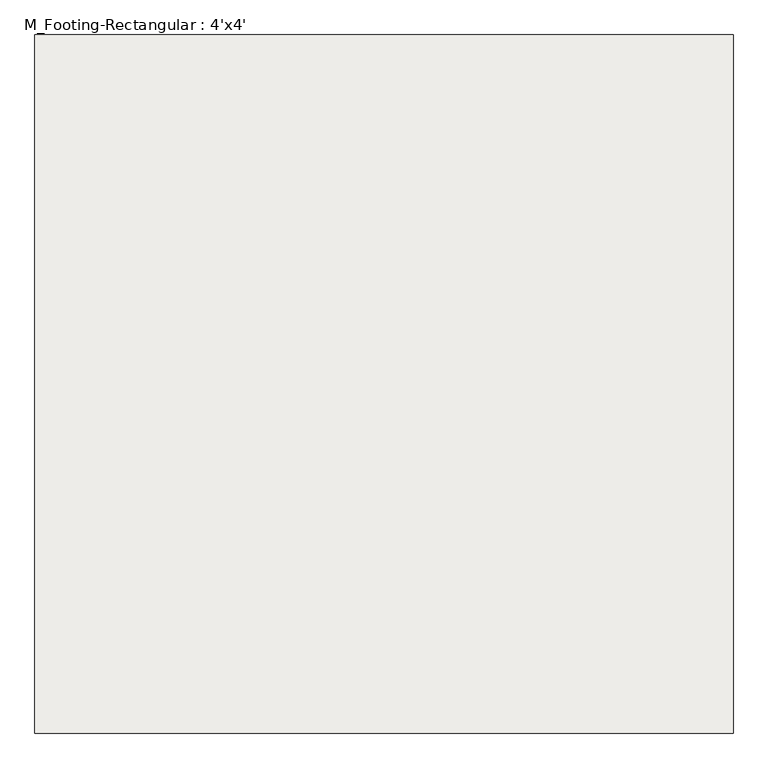
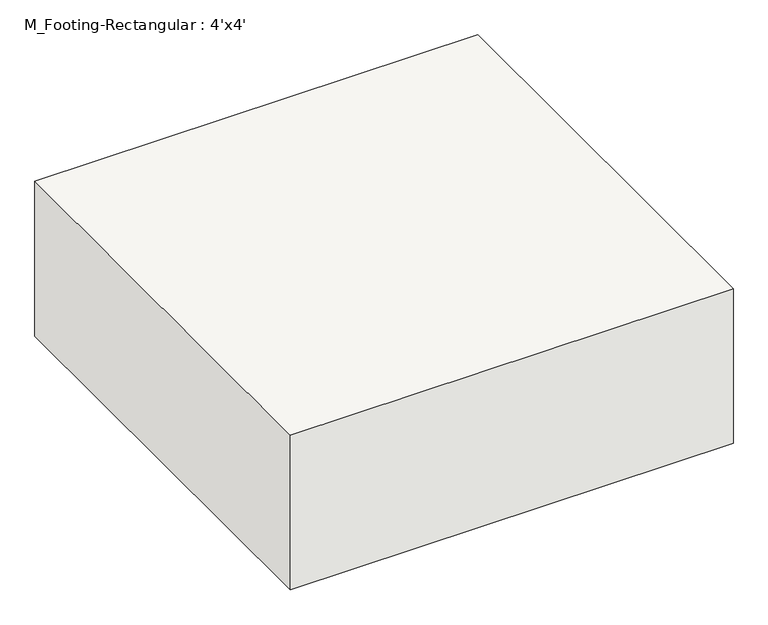
"""IFC4 building model written with IfcOpenShell, lengths in millimetres: slab geometry, M_Footing-Rectangular : 4'x4'."""

from ifc_helpers import new_model, si_unit, frame, origin, place, context, project, spatial, polyline, outline, extrude, source, transform, mapped, element, save


def m_footing_rectangular_4_x4_72b13ef4(model_context):
    return source(origin(), model_context, "Body", "SweptSolid", [
        extrude(outline(polyline([(609.6, 609.6), (609.6, -609.6), (-609.6, -609.6), (-609.6, 609.6), (609.6, 609.6)])), frame((0.0, 0.0, -450.0), z_axis=(0.0, 0.0, 1.0), x_axis=(1.0, 0.0, 0.0)), (0.0, 0.0, 1.0), 450.0),
    ])


if __name__ == "__main__":
    model = new_model("IFC4")
    model_context = context("Model", 3, world=origin())
    ifc_project = project(units=[si_unit("LENGTHUNIT", "METRE", prefix="MILLI")], contexts=[model_context])
    site = spatial("IfcSite", under=ifc_project)
    building = spatial("IfcBuilding", under=site)
    placement = place(None, origin())
    m_footing_rectangular_4_x4_shape = m_footing_rectangular_4_x4_72b13ef4(model_context)
    element("IfcSlab", 1, ObjectType="M_Footing-Rectangular : 4'x4'", at=placement, inside=building, context=model_context, shape_type="MappedRepresentation", body=[
        mapped(m_footing_rectangular_4_x4_shape, transform((0.0, 0.0, 0.0), x_axis=(1.0, 0.0, 0.0), y_axis=(0.0, 1.0, 0.0), z_axis=(0.0, 0.0, 1.0))),
    ])
    save(model, "model.ifc")

# Revit data of these elements
# Type "M_Footing-Rectangular : 4'x4'"
#   Width = 4' - 0"
#   Length = 4' - 0"
#   Foundation Thickness = 1' - 5.71654"
#   Structural Material [instance default] = Concrete, Cast-in-Place gray
#   Assembly Code = ""
# Element 1 (IfcSlab, "M_Footing-Rectangular : 4'x4'")
#   Materials on its faces: "Concrete, Cast-in-Place gray"
# Materials
#   "Concrete, Cast-in-Place gray": class "Concrete", colour RGB 192 192 192, transparency 0, Description = "Cast-in-place concrete", Cost = 0
